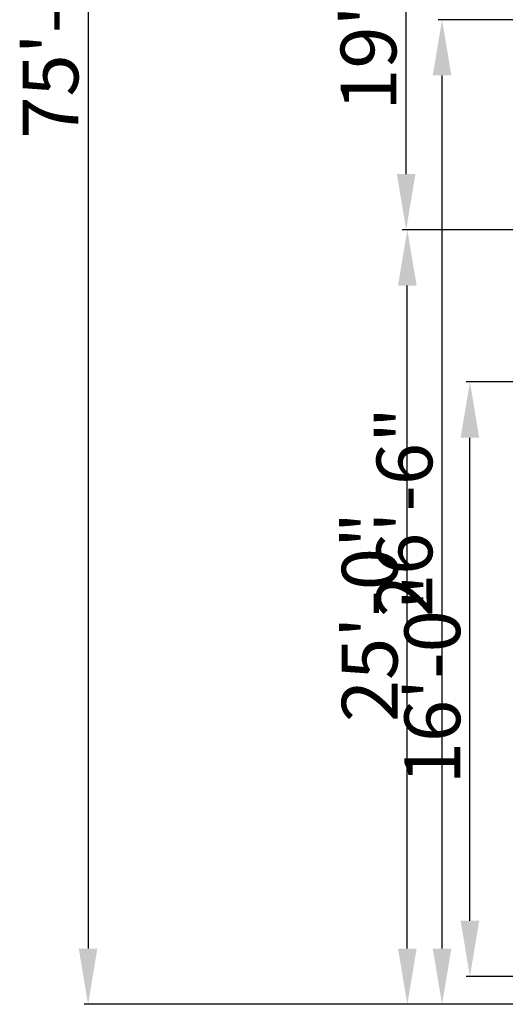
# Model space of a CAD drawing. Units: inches. Extents: x 2043 to 3177, y 1429 to 2563.
# Tile 2 of 14: x 2043 to 2200, y 1634 to 1952. Entities that reach past the tile are written whole.
import ezdxf

# ---------------------------------------------------------------- set-up
doc = ezdxf.new("R2010")
doc.units = ezdxf.units.IN
doc.layers.add('A-ANNO-DIMS', color=2, linetype='Continuous', lineweight=13)
doc.styles.get("Standard").update_dxf_attribs({"font": 'arial.ttf'})
doc.dimstyles.new('ISO-25', dxfattribs={"dimtxt": 18, "dimasz": 18, "dimexe": 1.25, "dimexo": 0.625, "dimtad": 1, "dimlunit": 3, "dimtxsty": 'Standard', "dimcen": 2.5, "dimadec": 0, "dimazin": 0, "dimtfac": 1, "dimtmove": 0, "dimatfit": 3, "dimfxl": 1, "dimarcsym": 0})

# ---------------------------------------------------------------- blocks, each defined once
blk = doc.blocks.new('*D25')
at = {"layer": 'A-ANNO-DIMS', "color": 0, "lineweight": -2, "transparency": 16777216}
for p, q in [((2233.12, 1884.52), (2167.18, 1884.52)), ((2168.43, 1652.39), (2168.43, 1866.52)), ((2233.12, 1634.39), (2167.18, 1634.39))]:
    blk.add_line(p, q, dxfattribs=at)
at = {"layer": 'A-ANNO-DIMS', "color": 0, "transparency": 16777216}
for points in [[(2165.43, 1866.52), (2171.43, 1866.52), (2168.43, 1884.52)], [(2165.43, 1652.39), (2171.43, 1652.39), (2168.43, 1634.39)]]:
    blk.add_solid(points, dxfattribs=at)
at = {"layer": 'Defpoints', "color": 0, "transparency": 16777216}
for p in [(2168.43, 1884.52), (2233.74, 1884.52), (2233.74, 1634.39)]:
    blk.add_point(p, dxfattribs=at)
at = {"layer": 'A-ANNO-DIMS', "color": 0, "transparency": 16777216, "insert": (2158.61, 1759.46), "char_height": 18, "attachment_point": 5, "rotation": 90}
blk.add_mtext('25\'-0"', dxfattribs=at)
blk = doc.blocks.new('*D26')
at = {"layer": 'A-ANNO-DIMS', "color": 0, "lineweight": -2, "transparency": 16777216}
for p, q in [((2233.12, 2029.27), (2166.79, 2029.27)), ((2168.04, 1902.52), (2168.04, 2011.27)), ((2233.12, 1884.52), (2166.79, 1884.52))]:
    blk.add_line(p, q, dxfattribs=at)
at = {"layer": 'A-ANNO-DIMS', "color": 0, "transparency": 16777216}
for points in [[(2165.04, 2011.27), (2171.04, 2011.27), (2168.04, 2029.27)], [(2165.04, 1902.52), (2171.04, 1902.52), (2168.04, 1884.52)]]:
    blk.add_solid(points, dxfattribs=at)
at = {"layer": 'Defpoints', "color": 0, "transparency": 16777216}
for p in [(2168.04, 2029.27), (2233.74, 2029.27), (2233.74, 1884.52)]:
    blk.add_point(p, dxfattribs=at)
at = {"layer": 'A-ANNO-DIMS', "color": 0, "transparency": 16777216, "insert": (2158.23, 1956.89), "char_height": 18, "attachment_point": 5, "rotation": 90}
blk.add_mtext('19\'-0"', dxfattribs=at)
blk = doc.blocks.new('*D28')
at = {"layer": 'A-ANNO-DIMS', "color": 0, "lineweight": -2, "transparency": 16777216}
for p, q in [((2233.12, 2261.39), (2064.1, 2261.39)), ((2065.35, 2243.39), (2065.35, 1652.39)), ((2233.12, 1634.39), (2064.1, 1634.39))]:
    blk.add_line(p, q, dxfattribs=at)
at = {"layer": 'A-ANNO-DIMS', "color": 0, "transparency": 16777216}
for points in [[(2062.35, 2243.39), (2068.35, 2243.39), (2065.35, 2261.39)], [(2062.35, 1652.39), (2068.35, 1652.39), (2065.35, 1634.39)]]:
    blk.add_solid(points, dxfattribs=at)
at = {"layer": 'Defpoints', "color": 0, "transparency": 16777216}
for p in [(2233.74, 2261.39), (2065.35, 1634.39), (2233.74, 1634.39)]:
    blk.add_point(p, dxfattribs=at)
at = {"layer": 'A-ANNO-DIMS', "color": 0, "transparency": 16777216, "insert": (2055.54, 1947.89), "char_height": 18, "attachment_point": 5, "rotation": 90}
blk.add_mtext('75\'-0"', dxfattribs=at)
blk = doc.blocks.new('*D74')
at = {"layer": 'A-ANNO-DIMS', "color": 0, "lineweight": -2, "transparency": 16777216}
for p, q in [((2242.12, 1952.39), (2178.39, 1952.39)), ((2179.64, 1652.39), (2179.64, 1934.39)), ((2233.12, 1634.39), (2178.39, 1634.39))]:
    blk.add_line(p, q, dxfattribs=at)
at = {"layer": 'A-ANNO-DIMS', "color": 0, "transparency": 16777216}
for points in [[(2176.64, 1934.39), (2182.64, 1934.39), (2179.64, 1952.39)], [(2176.64, 1652.39), (2182.64, 1652.39), (2179.64, 1634.39)]]:
    blk.add_solid(points, dxfattribs=at)
at = {"layer": 'Defpoints', "color": 0, "transparency": 16777216}
for p in [(2179.64, 1952.39), (2242.74, 1952.39), (2233.74, 1634.39)]:
    blk.add_point(p, dxfattribs=at)
at = {"layer": 'A-ANNO-DIMS', "color": 0, "transparency": 16777216, "insert": (2169.83, 1793.39), "char_height": 18, "attachment_point": 5, "rotation": 90}
blk.add_mtext('26\'-6"', dxfattribs=at)
blk = doc.blocks.new('*D76')
at = {"layer": 'A-ANNO-DIMS', "color": 0, "lineweight": -2, "transparency": 16777216}
for p, q in [((2242.12, 1835.39), (2187.39, 1835.39)), ((2188.64, 1661.39), (2188.64, 1817.39)), ((2242.12, 1643.39), (2187.39, 1643.39))]:
    blk.add_line(p, q, dxfattribs=at)
at = {"layer": 'A-ANNO-DIMS', "color": 0, "transparency": 16777216}
for points in [[(2185.64, 1817.39), (2191.64, 1817.39), (2188.64, 1835.39)], [(2185.64, 1661.39), (2191.64, 1661.39), (2188.64, 1643.39)]]:
    blk.add_solid(points, dxfattribs=at)
at = {"layer": 'Defpoints', "color": 0, "transparency": 16777216}
for p in [(2188.64, 1835.39), (2242.74, 1835.39), (2242.74, 1643.39)]:
    blk.add_point(p, dxfattribs=at)
at = {"layer": 'A-ANNO-DIMS', "color": 0, "transparency": 16777216, "insert": (2178.83, 1739.39), "char_height": 18, "attachment_point": 5, "rotation": 90}
blk.add_mtext('16\'-0"', dxfattribs=at)

msp = doc.modelspace()

# ---------------------------------------------------------------- dimensions: what is measured, and where the dimension line sits
at = {"layer": 'A-ANNO-DIMS'}
for base, p1, p2, text, picture, middle in [((2065.352, 1634.393), (2233.745, 2261.393), (2233.745, 1634.393), '75\'-0"', '*D28', (2055.537, 1947.893)), ((2168.041, 2029.268), (2233.745, 1884.518), (2233.745, 2029.268), '19\'-0"', '*D26', (2158.225, 1956.893)), ((2168.43, 1884.518), (2233.745, 1634.393), (2233.745, 1884.518), '25\'-0"', '*D25', (2158.615, 1759.456))]:
    dim = msp.add_linear_dim(base=base, p1=p1, p2=p2, angle=90, text=text, dimstyle='ISO-25', override={"dimclrd": 0, "dimclre": 0, "dimclrt": 0}, dxfattribs=at)
    dim.commit()
    dim.dimension.update_dxf_attribs({"geometry": picture, "text_midpoint": middle})
for base, p1, p2, picture, middle in [((2179.645, 1952.393), (2233.745, 1634.393), (2242.745, 1952.393), '*D74', (2169.829, 1793.393)), ((2188.645, 1835.393), (2242.745, 1643.393), (2242.745, 1835.393), '*D76', (2178.829, 1739.393))]:
    dim = msp.add_linear_dim(base=base, p1=p1, p2=p2, angle=90, dimstyle='ISO-25', override={"dimdec": 1, "dimlfac": 1, "dimrnd": 0, "dimzin": 1, "dimdsep": 46, "dimlunit": 4, "dimfrac": 2}, dxfattribs=at)
    dim.commit()
    dim.dimension.update_dxf_attribs({"geometry": picture, "text_midpoint": middle})

doc.saveas('drawing.dxf')
